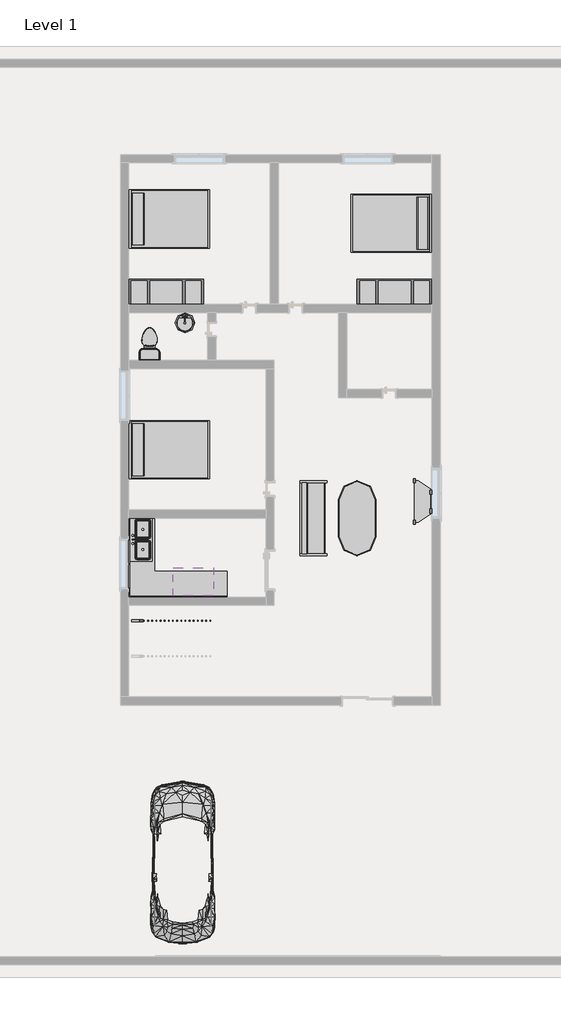
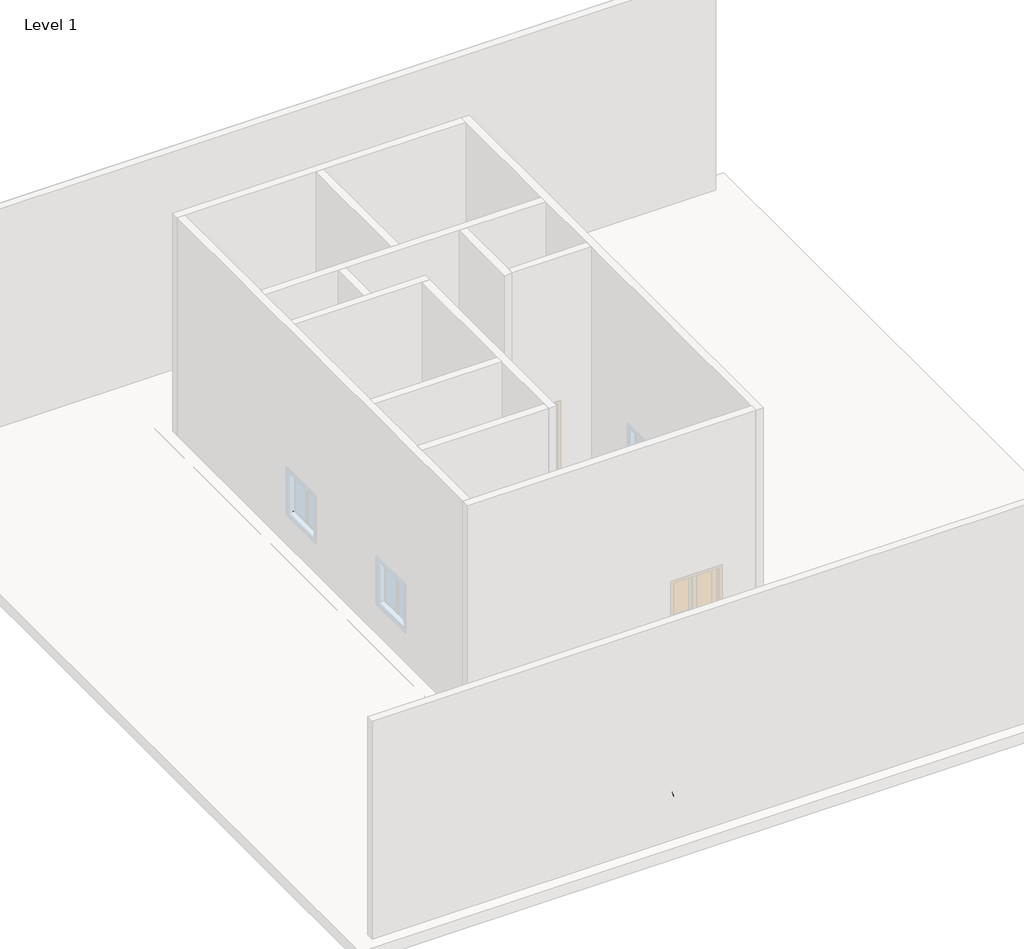
# One storey, part 3 of 3: 9 furniture elements, 3 flow terminals, 2 proxies, 1 railing.
"""IFC4 building model written with IfcOpenShell, lengths in millimetres."""

from ifc_helpers import new_model, si_unit, frame, origin, place, context, project, spatial, polyline, outline, extrude, faceted_brep, transform, mapped, element, save
from components import proxy_bb1e6e30, rpc_beetle_rpc_beetle_3ce7ba48, flow_terminal_a53be723, flow_terminal_d49f872f, toilet_domestic_3d_toilet_domestic_3d_f7549cf7, toilet_domestic_3d_toilet_domestic_3d_183bbd19, furniture_096e7f55, furniture_2f8694d0, furniture_cf0b6580, furniture_a4ffab56, tv_stand_tv_stand_6ce107e5, furniture_2c34a4f9

model = new_model("IFC4")

# Units and contexts
model_context = context("Model", 3, world=origin())
ifc_project = project(units=[si_unit("LENGTHUNIT", "METRE", prefix="MILLI")], contexts=[model_context])

# Site, building, storey
site = spatial("IfcSite", under=ifc_project)
building = spatial("IfcBuilding", under=site)
storey = spatial("IfcBuildingStorey", under=building, Name="Level 1", Elevation=0.0)

# Proxies
placement = place(None, origin())
proxy_shape = proxy_bb1e6e30(model_context)
element("IfcBuildingElementProxy", 1, Name="Cook Top-4 Unit : 36\" x 20\"", ObjectType="Cook Top-4 Unit : 36\" x 20\"", at=placement, inside=storey, context=model_context, shape_type="MappedRepresentation", body=[
    mapped(proxy_shape, transform((-9322.8260462, -2343.9818688, 914.4), x_axis=(1.0, 0.0, 0.0), y_axis=(0.0, 1.0, 0.0), z_axis=(0.0, 0.0, 1.0))),
])
rpc_beetle_rpc_beetle_shape = rpc_beetle_rpc_beetle_3ce7ba48(model_context)
element("IfcBuildingElementProxy", 2, Name="RPC Beetle : RPC Beetle", ObjectType="RPC Beetle : RPC Beetle", at=placement, inside=storey, context=model_context, shape_type="MappedRepresentation", body=[
    mapped(rpc_beetle_rpc_beetle_shape, transform((-9576.8260462, -10446.5818688, 0.0), x_axis=(1.0, 0.0, 0.0), y_axis=(0.0, 1.0, 0.0), z_axis=(0.0, 0.0, 1.0))),
])

# Flow terminals
flow_terminal_shape = flow_terminal_a53be723(model_context)
element("IfcFlowTerminal", 3, ObjectType="Sink Kitchen-Double : 42\" x 21\"", at=placement, inside=storey, context=model_context, shape_type="MappedRepresentation", body=[
    mapped(flow_terminal_shape, transform((-10590.4806451, -1330.9711094, 0.0), x_axis=(0.0, 1.0000000000000002, 0.0), y_axis=(-1.0000000000000002, 0.0, 0.0), z_axis=(0.0, 0.0, 1.0))),
])
flow_terminal_2_shape = flow_terminal_d49f872f(model_context)
element("IfcFlowTerminal", 4, ObjectType="Sink Vanity-Round : 19\" x 19\"", at=placement, inside=storey, context=model_context, shape_type="MappedRepresentation", body=[
    mapped(flow_terminal_2_shape, transform((-9622.6777868, 3894.5707398, 0.0), x_axis=(1.0, 0.0, 0.0), y_axis=(0.0, 1.0, 0.0), z_axis=(0.0, 0.0, 1.0))),
])
toilet_domestic_3d_toilet_domestic_3d_shape = toilet_domestic_3d_toilet_domestic_3d_f7549cf7(model_context)
toilet_domestic_3d_toilet_domestic_3d_2_shape = toilet_domestic_3d_toilet_domestic_3d_183bbd19(model_context)
element("IfcFlowTerminal", 5, ObjectType="Toilet-Domestic-3D : Toilet-Domestic-3D", at=placement, inside=storey, context=model_context, shape_type="MappedRepresentation", body=[
    mapped(toilet_domestic_3d_toilet_domestic_3d_shape, transform((-10389.6260462, 3560.9141586, 0.0), x_axis=(-1.0000000000000002, 0.0, 0.0), y_axis=(0.0, -1.0000000000000002, 0.0), z_axis=(0.0, 0.0, 1.0))),
    mapped(toilet_domestic_3d_toilet_domestic_3d_2_shape, transform((-10389.6260462, 3560.9141586, 0.0), x_axis=(-1.0000000000000002, 0.0, 0.0), y_axis=(0.0, -1.0000000000000002, 0.0), z_axis=(0.0, 0.0, 1.0))),
])

# Furniture
furniture_shape = furniture_096e7f55(model_context)
element("IfcFurniture", 6, ObjectType="Bed-Shaker : Double 56\" x 78\"", at=placement, inside=storey, context=model_context, shape_type="MappedRepresentation", body=[
    mapped(furniture_shape, transform((-10897.6260462, 6539.6681312, 0.0), x_axis=(0.0, 1.0000000000000002, 0.0), y_axis=(-1.0000000000000002, 0.0, 0.0), z_axis=(0.0, 0.0, 1.0))),
])
element("IfcFurniture", 7, ObjectType="Bed-Shaker : Double 56\" x 78\"", at=placement, inside=storey, context=model_context, shape_type="MappedRepresentation", body=[
    mapped(furniture_shape, transform((-3480.8260462, 6399.9681312, 0.0), x_axis=(0.0, -1.0000000000000004, 0.0), y_axis=(1.0000000000000004, 0.0, 0.0), z_axis=(0.0, 0.0, 1.0))),
])
element("IfcFurniture", 8, ObjectType="Bed-Shaker : Double 56\" x 78\"", at=placement, inside=storey, context=model_context, shape_type="MappedRepresentation", body=[
    mapped(furniture_shape, transform((-10897.6260462, 900.8681312, 0.0), x_axis=(0.0, 1.0000000000000004, 0.0), y_axis=(-1.0000000000000004, 0.0, 0.0), z_axis=(0.0, 0.0, 1.0))),
])
furniture_2_shape = furniture_2f8694d0(model_context)
element("IfcFurniture", 9, ObjectType="Counter Top-L Shaped w Sink : 24\" Depth", at=placement, inside=storey, context=model_context, shape_type="MappedRepresentation", body=[
    mapped(furniture_2_shape, transform((-10897.6260462, -1524.5195737, 0.0), x_axis=(0.0, 1.0000000000000002, 0.0), y_axis=(-1.0000000000000002, 0.0, 0.0), z_axis=(0.0, 0.0, 1.0))),
])
furniture_3_shape = furniture_cf0b6580(model_context)
element("IfcFurniture", 10, ObjectType="Entertainment Center : 72\" x 72\" x 24\"", at=placement, inside=storey, context=model_context, shape_type="MappedRepresentation", body=[
    mapped(furniture_3_shape, transform((-4395.2260462, 5149.0181312, 0.0), x_axis=(1.0, 0.0, 0.0), y_axis=(0.0, 1.0, 0.0), z_axis=(0.0, 0.0, 1.0))),
])
element("IfcFurniture", 11, ObjectType="Entertainment Center : 72\" x 72\" x 24\"", at=placement, inside=storey, context=model_context, shape_type="MappedRepresentation", body=[
    mapped(furniture_3_shape, transform((-9983.2260462, 5149.0181312, 0.0), x_axis=(1.0, 0.0, 0.0), y_axis=(0.0, 1.0, 0.0), z_axis=(0.0, 0.0, 1.0))),
])
furniture_4_shape = furniture_a4ffab56(model_context)
element("IfcFurniture", 12, ObjectType="Sofa : 72\"", at=placement, inside=storey, context=model_context, shape_type="MappedRepresentation", body=[
    mapped(furniture_4_shape, transform((-6230.2719478, -864.9523606, 0.0), x_axis=(0.0, 1.0000000000000002, 0.0), y_axis=(-1.0000000000000002, 0.0, 0.0), z_axis=(0.0, 0.0, 1.0))),
])
tv_stand_tv_stand_shape = tv_stand_tv_stand_6ce107e5(model_context)
element("IfcFurniture", 13, ObjectType="TV Stand : TV Stand", at=placement, inside=storey, context=model_context, shape_type="MappedRepresentation", body=[
    mapped(tv_stand_tv_stand_shape, transform((-3480.8260462, -262.9938667, 914.4), x_axis=(0.0, -1.0000000000000013, 0.0), y_axis=(1.0000000000000013, 0.0, 0.0), z_axis=(0.0, 0.0, 1.0))),
])
furniture_5_shape = furniture_2c34a4f9(model_context)
element("IfcFurniture", 14, ObjectType="Table-Dining Oval : 36\" x 72\"", at=placement, inside=storey, context=model_context, shape_type="MappedRepresentation", body=[
    mapped(furniture_5_shape, transform((-5667.7244068, -392.7621967, 0.0), x_axis=(0.0, 1.0, 0.0), y_axis=(-1.0, 0.0, 0.0), z_axis=(0.0, 0.0, 1.0))),
])

# Railing
element("IfcRailing", 15, ObjectType="Handrail - Rectangular", at=placement, inside=storey, context=model_context, shape_type="SolidModel", body=[
    faceted_brep([(-10833.7253666, -3277.3709044, 1090.3093851), (-10833.7253666, -3277.3709044, 1031.5187374), (-10833.7253666, -3328.1709044, 1031.5187374), (-10833.7253666, -3328.1709044, 1090.3093851), (-7938.1253666, -3277.3709044, 2777.0666667), (-7924.4080881, -3277.3709044, 2726.2666667), (-7924.4080881, -3328.1709044, 2726.2666667), (-7938.1253666, -3328.1709044, 2777.0666667), (-6534.7753666, -3277.3709044, 2777.0666667), (-6534.7753666, -3277.3709044, 2726.2666667), (-6585.5753666, -3328.1709044, 2726.2666667), (-6585.5753666, -3328.1709044, 2777.0666667), (-6534.7753666, -4928.3709044, 2777.0666667), (-6534.7753666, -4928.3709044, 2726.2666667), (-6585.5753666, -4877.5709044, 2726.2666667), (-6585.5753666, -4877.5709044, 2777.0666667), (-7169.7753666, -4928.3709044, 2777.0666667), (-7183.967776, -4928.3709044, 2726.2666667), (-7183.967776, -4877.5709044, 2726.2666667), (-7169.7753666, -4877.5709044, 2777.0666667), (-9125.5753666, -4928.3709044, 3962.4), (-9125.5753666, -4877.5709044, 3962.4), (-9125.5753666, -4877.5709044, 3902.9985397), (-9125.5753666, -4928.3709044, 3902.9985397)], [[[0, 1, 2, 3]], [[1, 0, 4, 5]], [[2, 1, 5, 6]], [[3, 2, 6, 7]], [[0, 3, 7, 4]], [[5, 4, 8, 9]], [[6, 5, 9, 10]], [[7, 6, 10, 11]], [[4, 7, 11, 8]], [[9, 8, 12, 13]], [[10, 9, 13, 14]], [[11, 10, 14, 15]], [[8, 11, 15, 12]], [[13, 12, 16, 17]], [[14, 13, 17, 18]], [[15, 14, 18, 19]], [[12, 15, 19, 16]], [[20, 21, 22, 23]], [[17, 16, 20, 23]], [[18, 17, 23, 22]], [[19, 18, 22, 21]], [[16, 19, 21, 20]]]),
    extrude(outline(polyline([(3893.3773276, -9109.7003666), (2878.6666667, -9109.7003666), (2878.6666667, -9090.6503666), (3881.8318731, -9090.6503666), (3893.3773276, -9109.7003666)])), frame((0.0, -4912.4959044, 0.0), z_axis=(0.0, 1.0, 0.0), x_axis=(0.0, 0.0, 1.0)), (0.0, 0.0, 1.0), 19.05),
    extrude(outline(polyline([(3831.80157, -9008.1003666), (2878.6666667, -9008.1003666), (2878.6666667, -8989.0503666), (3820.2561155, -8989.0503666), (3831.80157, -9008.1003666)])), frame((0.0, -4912.4959044, 0.0), z_axis=(0.0, 1.0, 0.0), x_axis=(0.0, 0.0, 1.0)), (0.0, 0.0, 1.0), 19.05),
    extrude(outline(polyline([(3770.2258125, -8906.5003666), (2878.6666667, -8906.5003666), (2878.6666667, -8887.4503666), (3758.6803579, -8887.4503666), (3770.2258125, -8906.5003666)])), frame((0.0, -4912.4959044, 0.0), z_axis=(0.0, 1.0, 0.0), x_axis=(0.0, 0.0, 1.0)), (0.0, 0.0, 1.0), 19.05),
    extrude(outline(polyline([(3708.6500549, -8804.9003666), (2709.3333333, -8804.9003666), (2709.3333333, -8785.8503666), (3697.1046004, -8785.8503666), (3708.6500549, -8804.9003666)])), frame((0.0, -4912.4959044, 0.0), z_axis=(0.0, 1.0, 0.0), x_axis=(0.0, 0.0, 1.0)), (0.0, 0.0, 1.0), 19.05),
    extrude(outline(polyline([(3647.0742973, -8703.3003666), (2709.3333333, -8703.3003666), (2709.3333333, -8684.2503666), (3635.5288428, -8684.2503666), (3647.0742973, -8703.3003666)])), frame((0.0, -4912.4959044, 0.0), z_axis=(0.0, 1.0, 0.0), x_axis=(0.0, 0.0, 1.0)), (0.0, 0.0, 1.0), 19.05),
    extrude(outline(polyline([(3585.4985397, -8601.7003666), (2709.3333333, -8601.7003666), (2709.3333333, -8582.6503666), (3573.9530852, -8582.6503666), (3585.4985397, -8601.7003666)])), frame((0.0, -4912.4959044, 0.0), z_axis=(0.0, 1.0, 0.0), x_axis=(0.0, 0.0, 1.0)), (0.0, 0.0, 1.0), 19.05),
    extrude(outline(polyline([(3523.9227822, -8500.1003666), (2540.0, -8500.1003666), (2540.0, -8481.0503666), (3512.3773276, -8481.0503666), (3523.9227822, -8500.1003666)])), frame((0.0, -4912.4959044, 0.0), z_axis=(0.0, 1.0, 0.0), x_axis=(0.0, 0.0, 1.0)), (0.0, 0.0, 1.0), 19.05),
    extrude(outline(polyline([(3462.3470246, -8398.5003666), (2540.0, -8398.5003666), (2540.0, -8379.4503666), (3450.80157, -8379.4503666), (3462.3470246, -8398.5003666)])), frame((0.0, -4912.4959044, 0.0), z_axis=(0.0, 1.0, 0.0), x_axis=(0.0, 0.0, 1.0)), (0.0, 0.0, 1.0), 19.05),
    extrude(outline(polyline([(3400.771267, -8296.9003666), (2540.0, -8296.9003666), (2540.0, -8277.8503666), (3389.2258125, -8277.8503666), (3400.771267, -8296.9003666)])), frame((0.0, -4912.4959044, 0.0), z_axis=(0.0, 1.0, 0.0), x_axis=(0.0, 0.0, 1.0)), (0.0, 0.0, 1.0), 19.05),
    extrude(outline(polyline([(3339.1955094, -8195.3003666), (2370.6666667, -8195.3003666), (2370.6666667, -8176.2503666), (3327.6500549, -8176.2503666), (3339.1955094, -8195.3003666)])), frame((0.0, -4912.4959044, 0.0), z_axis=(0.0, 1.0, 0.0), x_axis=(0.0, 0.0, 1.0)), (0.0, 0.0, 1.0), 19.05),
    extrude(outline(polyline([(3277.6197519, -8093.7003666), (2370.6666667, -8093.7003666), (2370.6666667, -8074.6503666), (3266.0742973, -8074.6503666), (3277.6197519, -8093.7003666)])), frame((0.0, -4912.4959044, 0.0), z_axis=(0.0, 1.0, 0.0), x_axis=(0.0, 0.0, 1.0)), (0.0, 0.0, 1.0), 19.05),
    extrude(outline(polyline([(3216.0439943, -7992.1003666), (2201.3333333, -7992.1003666), (2201.3333333, -7973.0503666), (3204.4985397, -7973.0503666), (3216.0439943, -7992.1003666)])), frame((0.0, -4912.4959044, 0.0), z_axis=(0.0, 1.0, 0.0), x_axis=(0.0, 0.0, 1.0)), (0.0, 0.0, 1.0), 19.05),
    extrude(outline(polyline([(3154.4682367, -7890.5003666), (2201.3333333, -7890.5003666), (2201.3333333, -7871.4503666), (3142.9227822, -7871.4503666), (3154.4682367, -7890.5003666)])), frame((0.0, -4912.4959044, 0.0), z_axis=(0.0, 1.0, 0.0), x_axis=(0.0, 0.0, 1.0)), (0.0, 0.0, 1.0), 19.05),
    extrude(outline(polyline([(3092.8924791, -7788.9003666), (2201.3333333, -7788.9003666), (2201.3333333, -7769.8503666), (3081.3470246, -7769.8503666), (3092.8924791, -7788.9003666)])), frame((0.0, -4912.4959044, 0.0), z_axis=(0.0, 1.0, 0.0), x_axis=(0.0, 0.0, 1.0)), (0.0, 0.0, 1.0), 19.05),
    extrude(outline(polyline([(3031.3167216, -7687.3003666), (2032.0, -7687.3003666), (2032.0, -7668.2503666), (3019.771267, -7668.2503666), (3031.3167216, -7687.3003666)])), frame((0.0, -4912.4959044, 0.0), z_axis=(0.0, 1.0, 0.0), x_axis=(0.0, 0.0, 1.0)), (0.0, 0.0, 1.0), 19.05),
    extrude(outline(polyline([(2969.740964, -7585.7003666), (2032.0, -7585.7003666), (2032.0, -7566.6503666), (2958.1955094, -7566.6503666), (2969.740964, -7585.7003666)])), frame((0.0, -4912.4959044, 0.0), z_axis=(0.0, 1.0, 0.0), x_axis=(0.0, 0.0, 1.0)), (0.0, 0.0, 1.0), 19.05),
    extrude(outline(polyline([(2908.1652064, -7484.1003666), (2032.0, -7484.1003666), (2032.0, -7465.0503666), (2896.6197519, -7465.0503666), (2908.1652064, -7484.1003666)])), frame((0.0, -4912.4959044, 0.0), z_axis=(0.0, 1.0, 0.0), x_axis=(0.0, 0.0, 1.0)), (0.0, 0.0, 1.0), 19.05),
    extrude(outline(polyline([(2846.5894488, -7382.5003666), (1862.6666667, -7382.5003666), (1862.6666667, -7363.4503666), (2835.0439943, -7363.4503666), (2846.5894488, -7382.5003666)])), frame((0.0, -4912.4959044, 0.0), z_axis=(0.0, 1.0, 0.0), x_axis=(0.0, 0.0, 1.0)), (0.0, 0.0, 1.0), 19.05),
    extrude(outline(polyline([(2785.0136913, -7280.9003666), (1862.6666667, -7280.9003666), (1862.6666667, -7261.8503666), (2773.4682367, -7261.8503666), (2785.0136913, -7280.9003666)])), frame((0.0, -4912.4959044, 0.0), z_axis=(0.0, 1.0, 0.0), x_axis=(0.0, 0.0, 1.0)), (0.0, 0.0, 1.0), 19.05),
    extrude(outline(polyline([(-7058.6503666, -4912.4959044), (-7077.7003666, -4912.4959044), (-7077.7003666, -4893.4459044), (-7058.6503666, -4893.4459044), (-7058.6503666, -4912.4959044)])), frame((0.0, 0.0, 1862.6666667), z_axis=(0.0, 0.0, 1.0), x_axis=(1.0, 0.0, 0.0)), (0.0, 0.0, 1.0), 863.6),
    extrude(outline(polyline([(-6957.0503666, -4912.4959044), (-6976.1003666, -4912.4959044), (-6976.1003666, -4893.4459044), (-6957.0503666, -4893.4459044), (-6957.0503666, -4912.4959044)])), frame((0.0, 0.0, 1862.6666667), z_axis=(0.0, 0.0, 1.0), x_axis=(1.0, 0.0, 0.0)), (0.0, 0.0, 1.0), 863.6),
    extrude(outline(polyline([(-6855.4503666, -4912.4959044), (-6874.5003666, -4912.4959044), (-6874.5003666, -4893.4459044), (-6855.4503666, -4893.4459044), (-6855.4503666, -4912.4959044)])), frame((0.0, 0.0, 1862.6666667), z_axis=(0.0, 0.0, 1.0), x_axis=(1.0, 0.0, 0.0)), (0.0, 0.0, 1.0), 863.6),
    extrude(outline(polyline([(-6753.8503666, -4912.4959044), (-6772.9003666, -4912.4959044), (-6772.9003666, -4893.4459044), (-6753.8503666, -4893.4459044), (-6753.8503666, -4912.4959044)])), frame((0.0, 0.0, 1862.6666667), z_axis=(0.0, 0.0, 1.0), x_axis=(1.0, 0.0, 0.0)), (0.0, 0.0, 1.0), 863.6),
    extrude(outline(polyline([(-6652.2503666, -4912.4959044), (-6671.3003666, -4912.4959044), (-6671.3003666, -4893.4459044), (-6652.2503666, -4893.4459044), (-6652.2503666, -4912.4959044)])), frame((0.0, 0.0, 1862.6666667), z_axis=(0.0, 0.0, 1.0), x_axis=(1.0, 0.0, 0.0)), (0.0, 0.0, 1.0), 863.6),
    extrude(outline(polyline([(-6550.6503666, -4817.2459044), (-6550.6503666, -4836.2959044), (-6569.7003666, -4836.2959044), (-6569.7003666, -4817.2459044), (-6550.6503666, -4817.2459044)])), frame((0.0, 0.0, 1862.6666667), z_axis=(0.0, 0.0, 1.0), x_axis=(1.0, 0.0, 0.0)), (0.0, 0.0, 1.0), 863.6),
    extrude(outline(polyline([(-6550.6503666, -4715.6459044), (-6550.6503666, -4734.6959044), (-6569.7003666, -4734.6959044), (-6569.7003666, -4715.6459044), (-6550.6503666, -4715.6459044)])), frame((0.0, 0.0, 1862.6666667), z_axis=(0.0, 0.0, 1.0), x_axis=(1.0, 0.0, 0.0)), (0.0, 0.0, 1.0), 863.6),
    extrude(outline(polyline([(-6550.6503666, -4614.0459044), (-6550.6503666, -4633.0959044), (-6569.7003666, -4633.0959044), (-6569.7003666, -4614.0459044), (-6550.6503666, -4614.0459044)])), frame((0.0, 0.0, 1862.6666667), z_axis=(0.0, 0.0, 1.0), x_axis=(1.0, 0.0, 0.0)), (0.0, 0.0, 1.0), 863.6),
    extrude(outline(polyline([(-6550.6503666, -4512.4459044), (-6550.6503666, -4531.4959044), (-6569.7003666, -4531.4959044), (-6569.7003666, -4512.4459044), (-6550.6503666, -4512.4459044)])), frame((0.0, 0.0, 1862.6666667), z_axis=(0.0, 0.0, 1.0), x_axis=(1.0, 0.0, 0.0)), (0.0, 0.0, 1.0), 863.6),
    extrude(outline(polyline([(-6550.6503666, -4410.8459044), (-6550.6503666, -4429.8959044), (-6569.7003666, -4429.8959044), (-6569.7003666, -4410.8459044), (-6550.6503666, -4410.8459044)])), frame((0.0, 0.0, 1862.6666667), z_axis=(0.0, 0.0, 1.0), x_axis=(1.0, 0.0, 0.0)), (0.0, 0.0, 1.0), 863.6),
    extrude(outline(polyline([(-6550.6503666, -4309.2459044), (-6550.6503666, -4328.2959044), (-6569.7003666, -4328.2959044), (-6569.7003666, -4309.2459044), (-6550.6503666, -4309.2459044)])), frame((0.0, 0.0, 1862.6666667), z_axis=(0.0, 0.0, 1.0), x_axis=(1.0, 0.0, 0.0)), (0.0, 0.0, 1.0), 863.6),
    extrude(outline(polyline([(-6550.6503666, -4207.6459044), (-6550.6503666, -4226.6959044), (-6569.7003666, -4226.6959044), (-6569.7003666, -4207.6459044), (-6550.6503666, -4207.6459044)])), frame((0.0, 0.0, 1862.6666667), z_axis=(0.0, 0.0, 1.0), x_axis=(1.0, 0.0, 0.0)), (0.0, 0.0, 1.0), 863.6),
    extrude(outline(polyline([(-6550.6503666, -4106.0459044), (-6550.6503666, -4125.0959044), (-6569.7003666, -4125.0959044), (-6569.7003666, -4106.0459044), (-6550.6503666, -4106.0459044)])), frame((0.0, 0.0, 1862.6666667), z_axis=(0.0, 0.0, 1.0), x_axis=(1.0, 0.0, 0.0)), (0.0, 0.0, 1.0), 863.6),
    extrude(outline(polyline([(-6550.6503666, -4004.4459044), (-6550.6503666, -4023.4959044), (-6569.7003666, -4023.4959044), (-6569.7003666, -4004.4459044), (-6550.6503666, -4004.4459044)])), frame((0.0, 0.0, 1862.6666667), z_axis=(0.0, 0.0, 1.0), x_axis=(1.0, 0.0, 0.0)), (0.0, 0.0, 1.0), 863.6),
    extrude(outline(polyline([(-6550.6503666, -3902.8459044), (-6550.6503666, -3921.8959044), (-6569.7003666, -3921.8959044), (-6569.7003666, -3902.8459044), (-6550.6503666, -3902.8459044)])), frame((0.0, 0.0, 1862.6666667), z_axis=(0.0, 0.0, 1.0), x_axis=(1.0, 0.0, 0.0)), (0.0, 0.0, 1.0), 863.6),
    extrude(outline(polyline([(-6550.6503666, -3801.2459044), (-6550.6503666, -3820.2959044), (-6569.7003666, -3820.2959044), (-6569.7003666, -3801.2459044), (-6550.6503666, -3801.2459044)])), frame((0.0, 0.0, 1862.6666667), z_axis=(0.0, 0.0, 1.0), x_axis=(1.0, 0.0, 0.0)), (0.0, 0.0, 1.0), 863.6),
    extrude(outline(polyline([(-6550.6503666, -3699.6459044), (-6550.6503666, -3718.6959044), (-6569.7003666, -3718.6959044), (-6569.7003666, -3699.6459044), (-6550.6503666, -3699.6459044)])), frame((0.0, 0.0, 1862.6666667), z_axis=(0.0, 0.0, 1.0), x_axis=(1.0, 0.0, 0.0)), (0.0, 0.0, 1.0), 863.6),
    extrude(outline(polyline([(-6550.6503666, -3598.0459044), (-6550.6503666, -3617.0959044), (-6569.7003666, -3617.0959044), (-6569.7003666, -3598.0459044), (-6550.6503666, -3598.0459044)])), frame((0.0, 0.0, 1862.6666667), z_axis=(0.0, 0.0, 1.0), x_axis=(1.0, 0.0, 0.0)), (0.0, 0.0, 1.0), 863.6),
    extrude(outline(polyline([(-6550.6503666, -3496.4459044), (-6550.6503666, -3515.4959044), (-6569.7003666, -3515.4959044), (-6569.7003666, -3496.4459044), (-6550.6503666, -3496.4459044)])), frame((0.0, 0.0, 1862.6666667), z_axis=(0.0, 0.0, 1.0), x_axis=(1.0, 0.0, 0.0)), (0.0, 0.0, 1.0), 863.6),
    extrude(outline(polyline([(-6550.6503666, -3394.8459044), (-6550.6503666, -3413.8959044), (-6569.7003666, -3413.8959044), (-6569.7003666, -3394.8459044), (-6550.6503666, -3394.8459044)])), frame((0.0, 0.0, 1862.6666667), z_axis=(0.0, 0.0, 1.0), x_axis=(1.0, 0.0, 0.0)), (0.0, 0.0, 1.0), 863.6),
    extrude(outline(polyline([(-6626.8503666, -3293.2459044), (-6607.8003666, -3293.2459044), (-6607.8003666, -3312.2959044), (-6626.8503666, -3312.2959044), (-6626.8503666, -3293.2459044)])), frame((0.0, 0.0, 1862.6666667), z_axis=(0.0, 0.0, 1.0), x_axis=(1.0, 0.0, 0.0)), (0.0, 0.0, 1.0), 863.6),
    extrude(outline(polyline([(-6728.4503666, -3293.2459044), (-6709.4003666, -3293.2459044), (-6709.4003666, -3312.2959044), (-6728.4503666, -3312.2959044), (-6728.4503666, -3293.2459044)])), frame((0.0, 0.0, 1862.6666667), z_axis=(0.0, 0.0, 1.0), x_axis=(1.0, 0.0, 0.0)), (0.0, 0.0, 1.0), 863.6),
    extrude(outline(polyline([(-6830.0503666, -3293.2459044), (-6811.0003666, -3293.2459044), (-6811.0003666, -3312.2959044), (-6830.0503666, -3312.2959044), (-6830.0503666, -3293.2459044)])), frame((0.0, 0.0, 1862.6666667), z_axis=(0.0, 0.0, 1.0), x_axis=(1.0, 0.0, 0.0)), (0.0, 0.0, 1.0), 863.6),
    extrude(outline(polyline([(-6931.6503666, -3293.2459044), (-6912.6003666, -3293.2459044), (-6912.6003666, -3312.2959044), (-6931.6503666, -3312.2959044), (-6931.6503666, -3293.2459044)])), frame((0.0, 0.0, 1862.6666667), z_axis=(0.0, 0.0, 1.0), x_axis=(1.0, 0.0, 0.0)), (0.0, 0.0, 1.0), 863.6),
    extrude(outline(polyline([(-7033.2503666, -3293.2459044), (-7014.2003666, -3293.2459044), (-7014.2003666, -3312.2959044), (-7033.2503666, -3312.2959044), (-7033.2503666, -3293.2459044)])), frame((0.0, 0.0, 1862.6666667), z_axis=(0.0, 0.0, 1.0), x_axis=(1.0, 0.0, 0.0)), (0.0, 0.0, 1.0), 863.6),
    extrude(outline(polyline([(-7134.8503666, -3293.2459044), (-7115.8003666, -3293.2459044), (-7115.8003666, -3312.2959044), (-7134.8503666, -3312.2959044), (-7134.8503666, -3293.2459044)])), frame((0.0, 0.0, 1862.6666667), z_axis=(0.0, 0.0, 1.0), x_axis=(1.0, 0.0, 0.0)), (0.0, 0.0, 1.0), 863.6),
    extrude(outline(polyline([(-7236.4503666, -3293.2459044), (-7217.4003666, -3293.2459044), (-7217.4003666, -3312.2959044), (-7236.4503666, -3312.2959044), (-7236.4503666, -3293.2459044)])), frame((0.0, 0.0, 1862.6666667), z_axis=(0.0, 0.0, 1.0), x_axis=(1.0, 0.0, 0.0)), (0.0, 0.0, 1.0), 863.6),
    extrude(outline(polyline([(-7338.0503666, -3293.2459044), (-7319.0003666, -3293.2459044), (-7319.0003666, -3312.2959044), (-7338.0503666, -3312.2959044), (-7338.0503666, -3293.2459044)])), frame((0.0, 0.0, 1862.6666667), z_axis=(0.0, 0.0, 1.0), x_axis=(1.0, 0.0, 0.0)), (0.0, 0.0, 1.0), 863.6),
    extrude(outline(polyline([(-7439.6503666, -3293.2459044), (-7420.6003666, -3293.2459044), (-7420.6003666, -3312.2959044), (-7439.6503666, -3312.2959044), (-7439.6503666, -3293.2459044)])), frame((0.0, 0.0, 1862.6666667), z_axis=(0.0, 0.0, 1.0), x_axis=(1.0, 0.0, 0.0)), (0.0, 0.0, 1.0), 863.6),
    extrude(outline(polyline([(-7541.2503666, -3293.2459044), (-7522.2003666, -3293.2459044), (-7522.2003666, -3312.2959044), (-7541.2503666, -3312.2959044), (-7541.2503666, -3293.2459044)])), frame((0.0, 0.0, 1862.6666667), z_axis=(0.0, 0.0, 1.0), x_axis=(1.0, 0.0, 0.0)), (0.0, 0.0, 1.0), 863.6),
    extrude(outline(polyline([(-7642.8503666, -3293.2459044), (-7623.8003666, -3293.2459044), (-7623.8003666, -3312.2959044), (-7642.8503666, -3312.2959044), (-7642.8503666, -3293.2459044)])), frame((0.0, 0.0, 1862.6666667), z_axis=(0.0, 0.0, 1.0), x_axis=(1.0, 0.0, 0.0)), (0.0, 0.0, 1.0), 863.6),
    extrude(outline(polyline([(-7744.4503666, -3293.2459044), (-7725.4003666, -3293.2459044), (-7725.4003666, -3312.2959044), (-7744.4503666, -3312.2959044), (-7744.4503666, -3293.2459044)])), frame((0.0, 0.0, 1862.6666667), z_axis=(0.0, 0.0, 1.0), x_axis=(1.0, 0.0, 0.0)), (0.0, 0.0, 1.0), 863.6),
    extrude(outline(polyline([(-7846.0503666, -3293.2459044), (-7827.0003666, -3293.2459044), (-7827.0003666, -3312.2959044), (-7846.0503666, -3312.2959044), (-7846.0503666, -3293.2459044)])), frame((0.0, 0.0, 1862.6666667), z_axis=(0.0, 0.0, 1.0), x_axis=(1.0, 0.0, 0.0)), (0.0, 0.0, 1.0), 863.6),
    extrude(outline(polyline([(2683.1352423, -7998.4503666), (1693.3333333, -7998.4503666), (1693.3333333, -7979.4003666), (2694.2323297, -7979.4003666), (2683.1352423, -7998.4503666)])), frame((0.0, -3312.2959044, 0.0), z_axis=(0.0, 1.0, 0.0), x_axis=(0.0, 0.0, 1.0)), (0.0, 0.0, 1.0), 19.05),
    extrude(outline(polyline([(2623.9507763, -8100.0503666), (1693.3333333, -8100.0503666), (1693.3333333, -8081.0003666), (2635.0478636, -8081.0003666), (2623.9507763, -8100.0503666)])), frame((0.0, -3312.2959044, 0.0), z_axis=(0.0, 1.0, 0.0), x_axis=(0.0, 0.0, 1.0)), (0.0, 0.0, 1.0), 19.05),
    extrude(outline(polyline([(2564.7663102, -8201.6503666), (1693.3333333, -8201.6503666), (1693.3333333, -8182.6003666), (2575.8633976, -8182.6003666), (2564.7663102, -8201.6503666)])), frame((0.0, -3312.2959044, 0.0), z_axis=(0.0, 1.0, 0.0), x_axis=(0.0, 0.0, 1.0)), (0.0, 0.0, 1.0), 19.05),
    extrude(outline(polyline([(2505.5818442, -8303.2503666), (1655.5210356, -8303.2503666), (1655.5210356, -8284.2003666), (2516.6789316, -8284.2003666), (2505.5818442, -8303.2503666)])), frame((0.0, -3312.2959044, 0.0), z_axis=(0.0, 1.0, 0.0), x_axis=(0.0, 0.0, 1.0)), (0.0, 0.0, 1.0), 19.05),
    extrude(outline(polyline([(2446.3973782, -8404.8503666), (1524.0, -8404.8503666), (1524.0, -8385.8003666), (2457.4944656, -8385.8003666), (2446.3973782, -8404.8503666)])), frame((0.0, -3312.2959044, 0.0), z_axis=(0.0, 1.0, 0.0), x_axis=(0.0, 0.0, 1.0)), (0.0, 0.0, 1.0), 19.05),
    extrude(outline(polyline([(2387.2129122, -8506.4503666), (1524.0, -8506.4503666), (1524.0, -8487.4003666), (2398.3099996, -8487.4003666), (2387.2129122, -8506.4503666)])), frame((0.0, -3312.2959044, 0.0), z_axis=(0.0, 1.0, 0.0), x_axis=(0.0, 0.0, 1.0)), (0.0, 0.0, 1.0), 19.05),
    extrude(outline(polyline([(2328.0284462, -8608.0503666), (1354.6666667, -8608.0503666), (1354.6666667, -8589.0003666), (2339.1255336, -8589.0003666), (2328.0284462, -8608.0503666)])), frame((0.0, -3312.2959044, 0.0), z_axis=(0.0, 1.0, 0.0), x_axis=(0.0, 0.0, 1.0)), (0.0, 0.0, 1.0), 19.05),
    extrude(outline(polyline([(2268.8439802, -8709.6503666), (1354.6666667, -8709.6503666), (1354.6666667, -8690.6003666), (2279.9410675, -8690.6003666), (2268.8439802, -8709.6503666)])), frame((0.0, -3312.2959044, 0.0), z_axis=(0.0, 1.0, 0.0), x_axis=(0.0, 0.0, 1.0)), (0.0, 0.0, 1.0), 19.05),
    extrude(outline(polyline([(2209.6595141, -8811.2503666), (1354.6666667, -8811.2503666), (1354.6666667, -8792.2003666), (2220.7566015, -8792.2003666), (2209.6595141, -8811.2503666)])), frame((0.0, -3312.2959044, 0.0), z_axis=(0.0, 1.0, 0.0), x_axis=(0.0, 0.0, 1.0)), (0.0, 0.0, 1.0), 19.05),
    extrude(outline(polyline([(2150.4750481, -8912.8503666), (1185.3333333, -8912.8503666), (1185.3333333, -8893.8003666), (2161.5721355, -8893.8003666), (2150.4750481, -8912.8503666)])), frame((0.0, -3312.2959044, 0.0), z_axis=(0.0, 1.0, 0.0), x_axis=(0.0, 0.0, 1.0)), (0.0, 0.0, 1.0), 19.05),
    extrude(outline(polyline([(2091.2905821, -9014.4503666), (1185.3333333, -9014.4503666), (1185.3333333, -8995.4003666), (2102.3876695, -8995.4003666), (2091.2905821, -9014.4503666)])), frame((0.0, -3312.2959044, 0.0), z_axis=(0.0, 1.0, 0.0), x_axis=(0.0, 0.0, 1.0)), (0.0, 0.0, 1.0), 19.05),
    extrude(outline(polyline([(2032.1061161, -9116.0503666), (1182.0453074, -9116.0503666), (1182.0453074, -9097.0003666), (2043.2032035, -9097.0003666), (2032.1061161, -9116.0503666)])), frame((0.0, -3312.2959044, 0.0), z_axis=(0.0, 1.0, 0.0), x_axis=(0.0, 0.0, 1.0)), (0.0, 0.0, 1.0), 19.05),
    extrude(outline(polyline([(1972.9216501, -9217.6503666), (1016.0, -9217.6503666), (1016.0, -9198.6003666), (1984.0187374, -9198.6003666), (1972.9216501, -9217.6503666)])), frame((0.0, -3312.2959044, 0.0), z_axis=(0.0, 1.0, 0.0), x_axis=(0.0, 0.0, 1.0)), (0.0, 0.0, 1.0), 19.05),
    extrude(outline(polyline([(1913.737184, -9319.2503666), (1016.0, -9319.2503666), (1016.0, -9300.2003666), (1924.8342714, -9300.2003666), (1913.737184, -9319.2503666)])), frame((0.0, -3312.2959044, 0.0), z_axis=(0.0, 1.0, 0.0), x_axis=(0.0, 0.0, 1.0)), (0.0, 0.0, 1.0), 19.05),
    extrude(outline(polyline([(1854.552718, -9420.8503666), (1004.4919094, -9420.8503666), (1004.4919094, -9401.8003666), (1865.6498054, -9401.8003666), (1854.552718, -9420.8503666)])), frame((0.0, -3312.2959044, 0.0), z_axis=(0.0, 1.0, 0.0), x_axis=(0.0, 0.0, 1.0)), (0.0, 0.0, 1.0), 19.05),
    extrude(outline(polyline([(1795.368252, -9522.4503666), (846.6666667, -9522.4503666), (846.6666667, -9503.4003666), (1806.4653394, -9503.4003666), (1795.368252, -9522.4503666)])), frame((0.0, -3312.2959044, 0.0), z_axis=(0.0, 1.0, 0.0), x_axis=(0.0, 0.0, 1.0)), (0.0, 0.0, 1.0), 19.05),
    extrude(outline(polyline([(1736.183786, -9624.0503666), (846.6666667, -9624.0503666), (846.6666667, -9605.0003666), (1747.2808734, -9605.0003666), (1736.183786, -9624.0503666)])), frame((0.0, -3312.2959044, 0.0), z_axis=(0.0, 1.0, 0.0), x_axis=(0.0, 0.0, 1.0)), (0.0, 0.0, 1.0), 19.05),
    extrude(outline(polyline([(1676.99932, -9725.6503666), (677.3333333, -9725.6503666), (677.3333333, -9706.6003666), (1688.0964073, -9706.6003666), (1676.99932, -9725.6503666)])), frame((0.0, -3312.2959044, 0.0), z_axis=(0.0, 1.0, 0.0), x_axis=(0.0, 0.0, 1.0)), (0.0, 0.0, 1.0), 19.05),
    extrude(outline(polyline([(1617.8148539, -9827.2503666), (677.3333333, -9827.2503666), (677.3333333, -9808.2003666), (1628.9119413, -9808.2003666), (1617.8148539, -9827.2503666)])), frame((0.0, -3312.2959044, 0.0), z_axis=(0.0, 1.0, 0.0), x_axis=(0.0, 0.0, 1.0)), (0.0, 0.0, 1.0), 19.05),
    extrude(outline(polyline([(1558.6303879, -9928.8503666), (677.3333333, -9928.8503666), (677.3333333, -9909.8003666), (1569.7274753, -9909.8003666), (1558.6303879, -9928.8503666)])), frame((0.0, -3312.2959044, 0.0), z_axis=(0.0, 1.0, 0.0), x_axis=(0.0, 0.0, 1.0)), (0.0, 0.0, 1.0), 19.05),
    extrude(outline(polyline([(1499.4459219, -10030.4503666), (508.0, -10030.4503666), (508.0, -10011.4003666), (1510.5430093, -10011.4003666), (1499.4459219, -10030.4503666)])), frame((0.0, -3312.2959044, 0.0), z_axis=(0.0, 1.0, 0.0), x_axis=(0.0, 0.0, 1.0)), (0.0, 0.0, 1.0), 19.05),
    extrude(outline(polyline([(1440.2614559, -10132.0503666), (508.0, -10132.0503666), (508.0, -10113.0003666), (1451.3585433, -10113.0003666), (1440.2614559, -10132.0503666)])), frame((0.0, -3312.2959044, 0.0), z_axis=(0.0, 1.0, 0.0), x_axis=(0.0, 0.0, 1.0)), (0.0, 0.0, 1.0), 19.05),
    extrude(outline(polyline([(1381.0769899, -10233.6503666), (508.0, -10233.6503666), (508.0, -10214.6003666), (1392.1740772, -10214.6003666), (1381.0769899, -10233.6503666)])), frame((0.0, -3312.2959044, 0.0), z_axis=(0.0, 1.0, 0.0), x_axis=(0.0, 0.0, 1.0)), (0.0, 0.0, 1.0), 19.05),
    extrude(outline(polyline([(1321.8925238, -10335.2503666), (338.6666667, -10335.2503666), (338.6666667, -10316.2003666), (1332.9896112, -10316.2003666), (1321.8925238, -10335.2503666)])), frame((0.0, -3312.2959044, 0.0), z_axis=(0.0, 1.0, 0.0), x_axis=(0.0, 0.0, 1.0)), (0.0, 0.0, 1.0), 19.05),
    extrude(outline(polyline([(1262.7080578, -10436.8503666), (338.6666667, -10436.8503666), (338.6666667, -10417.8003666), (1273.8051452, -10417.8003666), (1262.7080578, -10436.8503666)])), frame((0.0, -3312.2959044, 0.0), z_axis=(0.0, 1.0, 0.0), x_axis=(0.0, 0.0, 1.0)), (0.0, 0.0, 1.0), 19.05),
    extrude(outline(polyline([(1203.5235918, -10538.4503666), (338.6666667, -10538.4503666), (338.6666667, -10519.4003666), (1214.6206792, -10519.4003666), (1203.5235918, -10538.4503666)])), frame((0.0, -3312.2959044, 0.0), z_axis=(0.0, 1.0, 0.0), x_axis=(0.0, 0.0, 1.0)), (0.0, 0.0, 1.0), 19.05),
    extrude(outline(polyline([(1144.3391258, -10640.0503666), (169.3333333, -10640.0503666), (169.3333333, -10621.0003666), (1155.4362132, -10621.0003666), (1144.3391258, -10640.0503666)])), frame((0.0, -3312.2959044, 0.0), z_axis=(0.0, 1.0, 0.0), x_axis=(0.0, 0.0, 1.0)), (0.0, 0.0, 1.0), 19.05),
    extrude(outline(polyline([(1085.1546598, -10741.6503666), (169.3333333, -10741.6503666), (169.3333333, -10722.6003666), (1096.2517471, -10722.6003666), (1085.1546598, -10741.6503666)])), frame((0.0, -3312.2959044, 0.0), z_axis=(0.0, 1.0, 0.0), x_axis=(0.0, 0.0, 1.0)), (0.0, 0.0, 1.0), 19.05),
    extrude(outline(polyline([(-7160.2503666, -4912.4959044), (-7179.3003666, -4912.4959044), (-7179.3003666, -4893.4459044), (-7160.2503666, -4893.4459044), (-7160.2503666, -4912.4959044)])), frame((0.0, 0.0, 1862.6666667), z_axis=(0.0, 0.0, 1.0), x_axis=(1.0, 0.0, 0.0)), (0.0, 0.0, 1.0), 863.6),
    extrude(outline(polyline([(-6550.6503666, -4893.4459044), (-6550.6503666, -4912.4959044), (-6569.7003666, -4912.4959044), (-6569.7003666, -4893.4459044), (-6550.6503666, -4893.4459044)])), frame((0.0, 0.0, 1862.6666667), z_axis=(0.0, 0.0, 1.0), x_axis=(1.0, 0.0, 0.0)), (0.0, 0.0, 1.0), 863.6),
    extrude(outline(polyline([(-6569.7003666, -3293.2459044), (-6550.6503666, -3293.2459044), (-6550.6503666, -3312.2959044), (-6569.7003666, -3312.2959044), (-6569.7003666, -3293.2459044)])), frame((0.0, 0.0, 1862.6666667), z_axis=(0.0, 0.0, 1.0), x_axis=(1.0, 0.0, 0.0)), (0.0, 0.0, 1.0), 863.6),
    extrude(outline(polyline([(-7947.6503666, -3293.2459044), (-7928.6003666, -3293.2459044), (-7928.6003666, -3312.2959044), (-7947.6503666, -3312.2959044), (-7947.6503666, -3293.2459044)])), frame((0.0, 0.0, 1862.6666667), z_axis=(0.0, 0.0, 1.0), x_axis=(1.0, 0.0, 0.0)), (0.0, 0.0, 1.0), 863.6),
    extrude(outline(polyline([(3902.9985397, -9125.5753666), (2878.6666667, -9125.5753666), (2878.6666667, -9106.5253666), (3891.4530852, -9106.5253666), (3902.9985397, -9125.5753666)])), frame((0.0, -4912.4959044, 0.0), z_axis=(0.0, 1.0, 0.0), x_axis=(0.0, 0.0, 1.0)), (0.0, 0.0, 1.0), 19.05),
    extrude(outline(polyline([(1031.5187374, -10833.7253666), (169.3333333, -10833.7253666), (169.3333333, -10814.6753666), (1042.6158248, -10814.6753666), (1031.5187374, -10833.7253666)])), frame((0.0, -3312.2959044, 0.0), z_axis=(0.0, 1.0, 0.0), x_axis=(0.0, 0.0, 1.0)), (0.0, 0.0, 1.0), 19.05),
])

save(model, "model.ifc")

# Revit data of these elements
# Type "Cook Top-4 Unit : 36\" x 20\""
#   Assembly Code = "E1090400"
#   Depth = 2' - 0"
#   Width = 3' - 0"
#   Burner Material = Steel, Chrome Plated
#   Cooktop Material = Steel, Polished
#   Default Elevation = 0
# Type "RPC Beetle : RPC Beetle"
#   built-in parameter 1005195 = "RPC-16-0U6E-L4EG-ENH1-J3KF-SVEL-0TX4-C0"
#   Height = 0
# Type "Sink Kitchen-Double : 42\" x 21\""
#   Assembly Code = "D2010410"
#   Counter Height = 3' - 0"
#   Depth = 1' - 9"
#   Width = 3' - 6"
#   Faucet Material = Steel, Polished
#   Sink Material = Steel, Polished
#   Default Elevation = 0
# Type "Sink Vanity-Round : 19\" x 19\""
#   Assembly Code = "D2010400"
#   Top Of Counter = 2' - 7"
#   Basin Material = Porcelain, Linen
#   Faucet Material = Steel, Polished
#   Default Elevation = 0
# Type "Toilet-Domestic-3D : Toilet-Domestic-3D"
#   Assembly Code = "D2010110"
#   Toilet - Bowl/Basin Material = Porcelain, Linen
#   Toilet - Seat Material = Laminate, Linen, Matte
#   Default Elevation = 0
# Type "Bed-Shaker : Double 56\" x 78\""
#   Assembly Code = "E2020200"
#   Length = 6' - 6"
#   Width = 4' - 8"
#   Frame Material = Birch
#   Mattress Material = Linen, White
#   Default Elevation = 0
# Type "Counter Top-L Shaped w Sink : 24\" Depth"
#   Assembly Code = "C1030400"
#   Counter Thickness = 0' - 1 1/2"
#   Depth = 2' - 1"
#   Height = 3' - 0"
#   Length - Leg 1 [instance default] = 8' - 0"
#   Length - Leg 2 [instance default] = 6' - 0"
#   Sink Location [instance default] = 3' - 0"
#   Sink Location To Wall [instance default] = 0' - 6"
#   Sink Opening Depth [instance default] = 1' - 3"
#   Sink Opening Width [instance default] = 3' - 3"
#   Counter Top Material = none
#   Default Elevation = 0
# Type "Entertainment Center : 72\" x 72\" x 24\""
#   Assembly Code = "E2020200"
#   Center Width = 2' - 8"
#   Depth = 2' - 0"
#   Height = 6' - 0"
#   Width = 6' - 0"
#   Material = none
#   Default Elevation = 0
# Type "Sofa : 72\""
#   Assembly Code = "E2020200"
#   Width = 6' - 0"
#   Seat Material = Linen, Beige
#   Frame Material = Cherry
#   Default Elevation = 0
# Type "TV Stand : TV Stand"
#   Depth = 1' - 6"
#   Width = 3' - 8"
#   Height = 1' - 7 1/2"
#   Finish = Melamine - Gray
#   Default Elevation = 0
# Type "Table-Dining Oval : 36\" x 72\""
#   Assembly Code = "E2020200"
#   Length = 6' - 0"
#   Width = 3' - 0"
#   Base Material = Steel, Chrome Plated
#   Top Material = Glass - Clear, Grey
#   Default Elevation = 0
#   Description = (empty or 0)
# Type "Handrail - Rectangular"
#   Assembly Code = "C2010400"
#   built-in parameter 1008612 = 0.0416667 (stored number, unit not read)
#   built-in parameter 1008611 = 0.0416667 (stored number, unit not read)
#   built-in parameter 1008609 = 0.333333 (stored number, unit not read)
#   built-in parameter 1008604 = 0.166667 (stored number, unit not read)
#   built-in parameter 1008603 = 0.166667 (stored number, unit not read)
#   Railing Height = 3' - 0"
#   built-in parameter 1008630 = 2
#   built-in parameter 1008610 = 2
#   built-in parameter 1008618 = Baluster - Square : 3/4"
# Element 1 (IfcBuildingElementProxy, "Cook Top-4 Unit : 36\" x 20\"")
#   Phase Created = New Construction
#   Materials on its faces: "Steel, Chrome Plated", "Steel, Polished"
# Element 2 (IfcBuildingElementProxy, "RPC Beetle : RPC Beetle")
#   Phase Created = New Construction
# Element 3 (IfcFlowTerminal, "Sink Kitchen-Double : 42\" x 21\"")
#   Mark = "1"
#   Phase Created = New Construction
#   Materials on its faces: "Steel, Polished"
# Element 4 (IfcFlowTerminal, "Sink Vanity-Round : 19\" x 19\"")
#   Mark = "3"
#   Phase Created = New Construction
#   Materials on its faces: "Porcelain, Linen", "Steel, Polished"
# Element 5 (IfcFlowTerminal, "Toilet-Domestic-3D : Toilet-Domestic-3D")
#   Mark = "2"
#   Phase Created = New Construction
#   Materials on its faces: "Porcelain, Linen", "Laminate, Linen, Matte"
# Elements 6, 7, 8 (IfcFurniture, "Bed-Shaker : Double 56\" x 78\"")
#   Phase Created = New Construction
#   Materials on its faces: "Birch", "Linen, White"
# Element 9 (IfcFurniture, "Counter Top-L Shaped w Sink : 24\" Depth")
#   Sink Opening Width = 3' - 3"
#   Sink Opening Depth = 1' - 3"
#   Sink Location To Wall = 0' - 6"
#   Sink Location = 3' - 0"
#   Length - Leg 2 = 7' - 10.68053"
#   Length - Leg 1 = 6' - 4"
#   Phase Created = New Construction
#   Materials on its faces: "Counter Top"
# Elements 10, 11 (IfcFurniture, "Entertainment Center : 72\" x 72\" x 24\"")
#   Phase Created = New Construction
#   Materials on its faces: "Steel, Chrome Plated", "Glass - Clear, Grey"
# Element 12 (IfcFurniture, "Sofa : 72\"")
#   Phase Created = New Construction
#   Materials on its faces: "Cherry", "Linen, Beige"
# Element 13 (IfcFurniture, "TV Stand : TV Stand")
#   Phase Created = New Construction
#   Materials on its faces: "Melamine - Gray", "Glass - Shelves"
# Element 14 (IfcFurniture, "Table-Dining Oval : 36\" x 72\"")
#   Phase Created = New Construction
#   Materials on its faces: "Steel, Chrome Plated", "Glass - Clear, Grey"
# Element 15 (IfcRailing, "Handrail - Rectangular")
#   Phase Created = New Construction
# Materials
#   "Steel, Chrome Plated": class "Metal", colour RGB 17 17 17, transparency 0, Description = "Chromiuim plated steel", Cost = 0
#   "Steel, Polished": class "Metal", colour RGB 192 192 192, transparency 0, Description = "Polished steel", Cost = 0
#   "Porcelain, Linen": class "Ceramic", colour RGB 249 239 230, transparency 0, Description = "Porcelain, linen", Cost = 0
#   "Laminate, Linen, Matte": class "Plastic", colour RGB 249 239 230, transparency 0, Description = "Plastic Laminate - Linen, Matte", Cost = 0
#   "Birch": class "Wood", colour RGB 224 178 126, transparency 0, Description = "Betula Alleghaniensis", Cost = 0
#   "Linen, White": class "Textile", colour RGB 247 247 239, transparency 0, Description = "Linen, white", Cost = 0
#   "Linen, Beige": class "Textile", colour RGB 249 239 230, transparency 0, Description = "Linen, beige", Cost = 0
#   "Cherry": class "Wood", colour RGB 226 177 128, transparency 0, Description = "Prunus Serotina", Cost = 0
#   "Melamine - Gray": class "Wood", colour RGB 49 49 49, transparency 0
#   "Glass - Clear, Grey": class "Glass", colour RGB 252 255 255, transparency 0.64
#   "Counter Top": class "Wood", colour RGB 226 177 128, transparency 0
#   "Glass - Shelves": class "Glass", colour RGB 167 167 167, transparency 0.9
